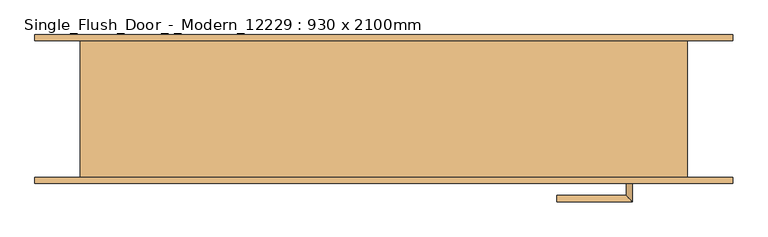
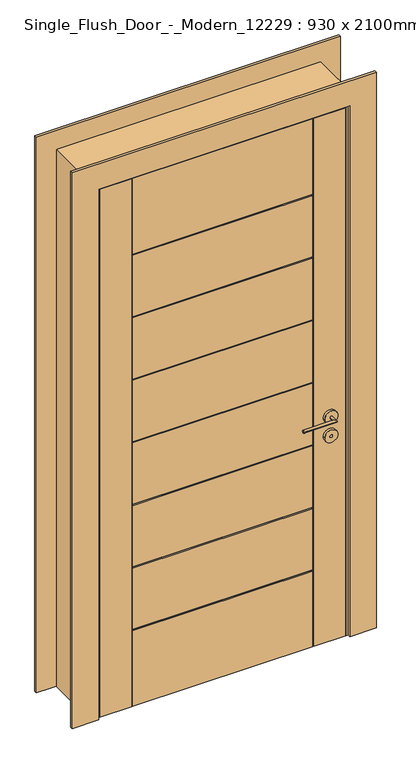
"""IFC4 building model written with IfcOpenShell, lengths in millimetres: door geometry, Single_Flush_Door_-_Modern_12229 : 930 x 2100mm."""

from ifc_helpers import new_model, si_unit, point, frame, frame_2d, origin, place, context, project, spatial, polyline, circle_curve, ellipse_curve, trimmed, segment, composite_curve, outline, extrude, faceted_brep, source, transform, mapped, element, save
from ifc_brep_helpers import plane_surface, cylinder_surface, advanced_brep


def single_flush_door_modern_12229_930_x_2100mm_fac4ccff(model_context):
    return source(origin(), model_context, "Body", "SolidModel", [
        extrude(outline(composite_curve([segment(trimmed(circle_curve(frame_2d((825.0, 405.0)), 25.0), [point((825.0, 380.0))], [point((825.0, 430.0))], False, "CARTESIAN"), True, "CONTINUOUS"), segment(trimmed(circle_curve(frame_2d((825.0, 405.0)), 25.0), [point((825.0, 430.0))], [point((825.0, 380.0))], False, "CARTESIAN"), True, "CONTINUOUS")], self_intersect=False), holes=[composite_curve([segment(trimmed(circle_curve(frame_2d((825.0, 405.0)), 5.0), [point((825.0, 400.0))], [point((825.0, 410.0))], True, "CARTESIAN"), True, "CONTINUOUS"), segment(trimmed(circle_curve(frame_2d((825.0, 405.0)), 5.0), [point((825.0, 410.0))], [point((825.0, 400.0))], True, "CARTESIAN"), True, "CONTINUOUS")], self_intersect=False)]), frame((0.0, -30.0, 0.0), z_axis=(0.0, 1.0, 0.0), x_axis=(0.0, 0.0, 1.0)), (0.0, 0.0, 1.0), 10.0),
        advanced_brep(
        [(410.0, -20.0, 900.0), (400.0, -20.0, 900.0), (410.0, 10.0, 900.0), (400.0, 0.0, 900.0), (285.0, 10.0, 900.0), (285.0, 0.0, 900.0)],
        [
            (0, 1, circle_curve(frame((405.0, -20.0, 900.0), z_axis=(0.0, -1.0, 0.0), x_axis=(-1.0, 0.0, 1.6983196031465473e-12)), 5.0)),
            (1, 0, circle_curve(frame((405.0, -20.0, 900.0), z_axis=(0.0, -1.0, 0.0), x_axis=(-1.0, 0.0, 1.6983196031465473e-12)), 5.0)),
            (0, 2),
            (2, 3, ellipse_curve(frame((405.0, 5.0, 900.0), z_axis=(0.7071067811869033, -0.7071067811861916, -1.2106711776242668e-12), x_axis=(-0.7071067811861915, -0.7071067811869034, 1.1911154383896718e-12)), 7.0710678, 5.0)),
            (3, 1),
            (3, 2, ellipse_curve(frame((405.0, 5.0, 900.0), z_axis=(0.7071067811869033, -0.7071067811861916, -1.2106711776242668e-12), x_axis=(-0.7071067811861915, -0.7071067811869034, 1.1911154383896718e-12)), 7.0710678, 5.0)),
            (4, 5, circle_curve(frame((285.0, 5.0, 900.0), z_axis=(-1.0, 0.0, 1.6983196031465471e-12), x_axis=(0.0, -1.0, 0.0)), 5.0)),
            (5, 4, circle_curve(frame((285.0, 5.0, 900.0), z_axis=(-1.0, 0.0, 1.6983196031465471e-12), x_axis=(0.0, -1.0, 0.0)), 5.0)),
            (2, 4),
            (5, 3),
        ],
        [
            plane_surface(frame((405.0, -20.0, 900.0), z_axis=(0.0, -1.0, 0.0), x_axis=(1.6983196031465542e-12, 0.0, 1.0))),
            cylinder_surface(frame((405.0, -20.0, 900.0), z_axis=(0.0, -1.0, 0.0), x_axis=(-1.0, 0.0, 1.6983196031465473e-12)), 5.0),
            plane_surface(frame((285.0, 5.0, 900.0), z_axis=(-1.0, 0.0, 1.6983196031465473e-12), x_axis=(1.6983196031465542e-12, 0.0, 1.0))),
            cylinder_surface(frame((405.0, 5.0, 900.0), z_axis=(1.0, 0.0, -1.6983196031465471e-12), x_axis=(0.0, -1.0, 0.0)), 5.0),
        ],
        [
            (0, [[1, 2]]),
            (1, [[-1, 3, 4, 5]]),
            (1, [[-2, -5, 6, -3]]),
            (2, [[7, 8]]),
            (3, [[-4, 9, -8, 10]]),
            (3, [[-6, -10, -7, -9]]),
        ],
    ),
        extrude(outline(composite_curve([segment(trimmed(circle_curve(frame_2d((900.0, 405.0)), 25.0), [point((900.0, 380.0))], [point((900.0, 430.0))], False, "CARTESIAN"), True, "CONTINUOUS"), segment(trimmed(circle_curve(frame_2d((900.0, 405.0)), 25.0), [point((900.0, 430.0))], [point((900.0, 380.0))], False, "CARTESIAN"), True, "CONTINUOUS")], self_intersect=False)), frame((0.0, -30.0, 0.0), z_axis=(0.0, 1.0, 0.0), x_axis=(0.0, 0.0, 1.0)), (0.0, 0.0, 1.0), 10.0),
        extrude(outline(composite_curve([segment(trimmed(circle_curve(frame_2d((825.0, 405.0)), 25.0), [point((825.0, 380.0))], [point((825.0, 430.0))], False, "CARTESIAN"), True, "CONTINUOUS"), segment(trimmed(circle_curve(frame_2d((825.0, 405.0)), 25.0), [point((825.0, 430.0))], [point((825.0, 380.0))], False, "CARTESIAN"), True, "CONTINUOUS")], self_intersect=False), holes=[composite_curve([segment(trimmed(circle_curve(frame_2d((825.0, 405.0)), 5.0), [point((825.0, 400.0))], [point((825.0, 410.0))], True, "CARTESIAN"), True, "CONTINUOUS"), segment(trimmed(circle_curve(frame_2d((825.0, 405.0)), 5.0), [point((825.0, 410.0))], [point((825.0, 400.0))], True, "CARTESIAN"), True, "CONTINUOUS")], self_intersect=False)]), frame((0.0, -122.5, 0.0), z_axis=(0.0, 1.0, 0.0), x_axis=(0.0, 0.0, 1.0)), (0.0, 0.0, 1.0), 10.0),
        advanced_brep(
        [(410.0, -122.5, 900.0), (400.0, -122.5, 900.0), (400.0, -142.5, 900.0), (410.0, -152.5, 900.0), (285.0, -152.5, 900.0), (285.0, -142.5, 900.0)],
        [
            (0, 1, circle_curve(frame((405.0, -122.5, 900.0), z_axis=(0.0, 1.0, 0.0), x_axis=(-1.0, 0.0, -1.9708679133145848e-12)), 5.0)),
            (1, 0, circle_curve(frame((405.0, -122.5, 900.0), z_axis=(0.0, 1.0, 0.0), x_axis=(-1.0, 0.0, -1.9708679133145848e-12)), 5.0)),
            (1, 2),
            (2, 3, ellipse_curve(frame((405.0, -147.5, 900.0), z_axis=(0.7071067811869033, 0.7071067811861916, 1.3838361967117316e-12), x_axis=(-0.7071067811861915, 0.7071067811869034, -1.4033919359437145e-12)), 7.0710678, 5.0)),
            (3, 0),
            (3, 2, ellipse_curve(frame((405.0, -147.5, 900.0), z_axis=(0.7071067811869033, 0.7071067811861916, 1.3838361967117316e-12), x_axis=(-0.7071067811861915, 0.7071067811869034, -1.4033919359437145e-12)), 7.0710678, 5.0)),
            (4, 5, circle_curve(frame((285.0, -147.5, 900.0), z_axis=(-1.0, 0.0, -1.9708679133145848e-12), x_axis=(0.0, 1.0, 0.0)), 5.0)),
            (5, 4, circle_curve(frame((285.0, -147.5, 900.0), z_axis=(-1.0, 0.0, -1.9708679133145848e-12), x_axis=(0.0, 1.0, 0.0)), 5.0)),
            (2, 5),
            (4, 3),
        ],
        [
            plane_surface(frame((405.0, -122.5, 900.0), z_axis=(0.0, 1.0, 0.0), x_axis=(-1.970867913314578e-12, 0.0, 1.0))),
            cylinder_surface(frame((405.0, -122.5, 900.0), z_axis=(0.0, 1.0, 0.0), x_axis=(-1.0, 0.0, -1.9708679133145848e-12)), 5.0),
            plane_surface(frame((285.0, -147.5, 900.0), z_axis=(-1.0, 0.0, -1.9708679133145848e-12), x_axis=(-1.970867913314578e-12, 0.0, 1.0))),
            cylinder_surface(frame((405.0, -147.5, 900.0), z_axis=(1.0, 0.0, 1.9708679133145848e-12), x_axis=(0.0, 1.0, 0.0)), 5.0),
        ],
        [
            (0, [[1, 2]]),
            (1, [[3, 4, 5, -2]]),
            (1, [[-5, 6, -3, -1]]),
            (2, [[7, 8]]),
            (3, [[9, -7, 10, -4]]),
            (3, [[-10, -8, -9, -6]]),
        ],
    ),
        extrude(outline(composite_curve([segment(trimmed(circle_curve(frame_2d((900.0, 405.0)), 25.0), [point((900.0, 380.0))], [point((900.0, 430.0))], False, "CARTESIAN"), True, "CONTINUOUS"), segment(trimmed(circle_curve(frame_2d((900.0, 405.0)), 25.0), [point((900.0, 430.0))], [point((900.0, 380.0))], False, "CARTESIAN"), True, "CONTINUOUS")], self_intersect=False)), frame((0.0, -122.5, 0.0), z_axis=(0.0, 1.0, 0.0), x_axis=(0.0, 0.0, 1.0)), (0.0, 0.0, 1.0), 10.0),
        extrude(outline(polyline([(2220.0, -575.0), (0.0, -575.0), (0.0, -475.0), (2120.0, -475.0), (2120.0, 475.0), (0.0, 475.0), (0.0, 575.0), (2220.0, 575.0), (2220.0, -575.0)])), frame((0.0, -122.5, 0.0), z_axis=(0.0, 1.0, 0.0), x_axis=(0.0, 0.0, 1.0)), (0.0, 0.0, 1.0), 10.0),
        extrude(outline(polyline([(2120.0, -475.0), (2120.0, 475.0), (0.0, 475.0), (0.0, 575.0), (2220.0, 575.0), (2220.0, -575.0), (0.0, -575.0), (0.0, -475.0), (2120.0, -475.0)])), frame((0.0, 112.5, 0.0), z_axis=(0.0, 1.0, 0.0), x_axis=(0.0, 0.0, 1.0)), (0.0, 0.0, 1.0), 10.0),
        faceted_brep([(-455.0, 112.5, 0.0), (-455.0, -30.0, 0.0), (-465.0, -30.0, 0.0), (-465.0, -112.5, 0.0), (-500.0, -112.5, 0.0), (-500.0, 112.5, 0.0), (-455.0, 112.5, 2100.0), (-455.0, -30.0, 2100.0), (-345.0, -30.0, 2100.0), (-340.0, -30.0, 2100.0), (340.0, -30.0, 2100.0), (345.0, -30.0, 2100.0), (455.0, -30.0, 2100.0), (455.0, -30.0, 0.0), (465.0, -30.0, 0.0), (465.0, -30.0, 2110.0), (345.0, -30.0, 2110.0), (340.0, -30.0, 2110.0), (-340.0, -30.0, 2110.0), (-345.0, -30.0, 2110.0), (-465.0, -30.0, 2110.0), (-465.0, -112.5, 2110.0), (-345.0, -112.5, 2110.0), (-340.0, -112.5, 2110.0), (340.0, -112.5, 2110.0), (345.0, -112.5, 2110.0), (465.0, -112.5, 2110.0), (465.0, -112.5, 0.0), (500.0, -112.5, 0.0), (500.0, -112.5, 2145.0), (-500.0, -112.5, 2145.0), (-500.0, 112.5, 2145.0), (500.0, 112.5, 2145.0), (500.0, 112.5, 0.0), (455.0, 112.5, 0.0), (455.0, 112.5, 2100.0)], [[[0, 1, 2, 3, 4, 5]], [[1, 0, 6, 7]], [[2, 1, 7, 8, 9, 10, 11, 12, 13, 14, 15, 16, 17, 18, 19, 20]], [[3, 2, 20, 21]], [[4, 3, 21, 22, 23, 24, 25, 26, 27, 28, 29, 30]], [[5, 4, 30, 31]], [[0, 5, 31, 32, 33, 34, 35, 6]], [[13, 12, 35, 34]], [[14, 13, 34, 33, 28, 27]], [[15, 14, 27, 26]], [[29, 28, 33, 32]], [[7, 6, 35, 12, 11, 10, 9, 8]], [[21, 20, 19, 18, 17, 16, 15, 26, 25, 24, 23, 22]], [[30, 29, 32, 31]]]),
        faceted_brep([(465.0, -112.5, 2110.0), (465.0, -30.0, 2110.0), (345.0, -30.0, 2110.0), (345.0, -35.0, 2110.0), (340.0, -35.0, 2110.0), (340.0, -30.0, 2110.0), (-340.0, -30.0, 2110.0), (-340.0, -35.0, 2110.0), (-345.0, -35.0, 2110.0), (-345.0, -30.0, 2110.0), (-465.0, -30.0, 2110.0), (-465.0, -112.5, 2110.0), (-345.0, -112.5, 2110.0), (-345.0, -107.5, 2110.0), (-340.0, -107.5, 2110.0), (-340.0, -112.5, 2110.0), (340.0, -112.5, 2110.0), (340.0, -107.5, 2110.0), (345.0, -107.5, 2110.0), (345.0, -112.5, 2110.0), (-465.0, -112.5, 0.0), (-465.0, -30.0, 0.0), (-345.0, -30.0, 0.0), (-345.0, -35.0, 0.0), (-340.0, -35.0, 0.0), (-340.0, -30.0, 0.0), (340.0, -30.0, 0.0), (340.0, -35.0, 0.0), (345.0, -35.0, 0.0), (345.0, -30.0, 0.0), (465.0, -30.0, 0.0), (465.0, -112.5, 0.0), (345.0, -112.5, 0.0), (345.0, -107.5, 0.0), (340.0, -107.5, 0.0), (340.0, -112.5, 0.0), (-340.0, -112.5, 0.0), (-340.0, -107.5, 0.0), (-345.0, -107.5, 0.0), (-345.0, -112.5, 0.0), (340.0, -30.0, 1807.5), (-340.0, -30.0, 1807.5), (-340.0, -30.0, 302.5), (340.0, -30.0, 302.5), (340.0, -30.0, 1802.5), (340.0, -30.0, 1557.5), (-340.0, -30.0, 1557.5), (-340.0, -30.0, 1802.5), (340.0, -30.0, 1552.5), (340.0, -30.0, 1307.5), (-340.0, -30.0, 1307.5), (-340.0, -30.0, 1552.5), (340.0, -30.0, 1302.5), (340.0, -30.0, 1057.5), (-340.0, -30.0, 1057.5), (-340.0, -30.0, 1302.5), (340.0, -30.0, 1052.5), (340.0, -30.0, 807.5), (-340.0, -30.0, 807.5), (-340.0, -30.0, 1052.5), (340.0, -30.0, 802.5), (340.0, -30.0, 557.5), (-340.0, -30.0, 557.5), (-340.0, -30.0, 802.5), (340.0, -30.0, 552.5), (340.0, -30.0, 307.5), (-340.0, -30.0, 307.5), (-340.0, -30.0, 552.5), (-340.0, -112.5, 1807.5), (340.0, -112.5, 1807.5), (340.0, -112.5, 302.5), (-340.0, -112.5, 302.5), (-340.0, -112.5, 1802.5), (-340.0, -112.5, 1557.5), (340.0, -112.5, 1557.5), (340.0, -112.5, 1802.5), (-340.0, -112.5, 1552.5), (-340.0, -112.5, 1307.5), (340.0, -112.5, 1307.5), (340.0, -112.5, 1552.5), (-340.0, -112.5, 1302.5), (-340.0, -112.5, 1057.5), (340.0, -112.5, 1057.5), (340.0, -112.5, 1302.5), (-340.0, -112.5, 1052.5), (-340.0, -112.5, 807.5), (340.0, -112.5, 807.5), (340.0, -112.5, 1052.5), (-340.0, -112.5, 802.5), (-340.0, -112.5, 557.5), (340.0, -112.5, 557.5), (340.0, -112.5, 802.5), (-340.0, -112.5, 552.5), (-340.0, -112.5, 307.5), (340.0, -112.5, 307.5), (340.0, -112.5, 552.5), (-340.0, -107.5, 302.5), (340.0, -107.5, 302.5), (340.0, -107.5, 1807.5), (-340.0, -107.5, 1807.5), (-340.0, -107.5, 1802.5), (340.0, -107.5, 1802.5), (340.0, -107.5, 1557.5), (-340.0, -107.5, 1557.5), (-340.0, -107.5, 1552.5), (340.0, -107.5, 1552.5), (340.0, -107.5, 1307.5), (-340.0, -107.5, 1307.5), (-340.0, -107.5, 1302.5), (340.0, -107.5, 1302.5), (340.0, -107.5, 1057.5), (-340.0, -107.5, 1057.5), (-340.0, -107.5, 1052.5), (340.0, -107.5, 1052.5), (340.0, -107.5, 807.5), (-340.0, -107.5, 807.5), (-340.0, -107.5, 802.5), (340.0, -107.5, 802.5), (340.0, -107.5, 557.5), (-340.0, -107.5, 557.5), (-340.0, -107.5, 552.5), (340.0, -107.5, 552.5), (340.0, -107.5, 307.5), (-340.0, -107.5, 307.5), (340.0, -35.0, 302.5), (-340.0, -35.0, 302.5), (-340.0, -35.0, 1807.5), (340.0, -35.0, 1807.5), (340.0, -35.0, 1557.5), (340.0, -35.0, 1802.5), (-340.0, -35.0, 1802.5), (-340.0, -35.0, 1557.5), (340.0, -35.0, 1307.5), (340.0, -35.0, 1552.5), (-340.0, -35.0, 1552.5), (-340.0, -35.0, 1307.5), (340.0, -35.0, 1057.5), (340.0, -35.0, 1302.5), (-340.0, -35.0, 1302.5), (-340.0, -35.0, 1057.5), (340.0, -35.0, 807.5), (340.0, -35.0, 1052.5), (-340.0, -35.0, 1052.5), (-340.0, -35.0, 807.5), (340.0, -35.0, 557.5), (340.0, -35.0, 802.5), (-340.0, -35.0, 802.5), (-340.0, -35.0, 557.5), (340.0, -35.0, 307.5), (340.0, -35.0, 552.5), (-340.0, -35.0, 552.5), (-340.0, -35.0, 307.5)], [[[0, 1, 2, 3, 4, 5, 6, 7, 8, 9, 10, 11, 12, 13, 14, 15, 16, 17, 18, 19]], [[20, 21, 22, 23, 24, 25, 26, 27, 28, 29, 30, 31, 32, 33, 34, 35, 36, 37, 38, 39]], [[1, 0, 31, 30]], [[6, 5, 40, 41]], [[26, 25, 42, 43]], [[1, 30, 29, 2]], [[21, 10, 9, 22]], [[44, 45, 46, 47]], [[48, 49, 50, 51]], [[52, 53, 54, 55]], [[56, 57, 58, 59]], [[60, 61, 62, 63]], [[64, 65, 66, 67]], [[11, 10, 21, 20]], [[16, 15, 68, 69]], [[36, 35, 70, 71]], [[31, 0, 19, 32]], [[11, 20, 39, 12]], [[72, 73, 74, 75]], [[76, 77, 78, 79]], [[80, 81, 82, 83]], [[84, 85, 86, 87]], [[88, 89, 90, 91]], [[92, 93, 94, 95]], [[13, 38, 37, 96, 97, 34, 33, 18, 17, 98, 99, 14], [100, 101, 102, 103], [104, 105, 106, 107], [108, 109, 110, 111], [112, 113, 114, 115], [116, 117, 118, 119], [120, 121, 122, 123]], [[15, 14, 99, 68]], [[37, 36, 71, 96]], [[73, 72, 100, 103]], [[77, 76, 104, 107]], [[81, 80, 108, 111]], [[85, 84, 112, 115]], [[89, 88, 116, 119]], [[93, 92, 120, 123]], [[38, 13, 12, 39]], [[18, 33, 32, 19]], [[17, 16, 69, 98]], [[35, 34, 97, 70]], [[75, 74, 102, 101]], [[79, 78, 106, 105]], [[83, 82, 110, 109]], [[87, 86, 114, 113]], [[91, 90, 118, 117]], [[95, 94, 122, 121]], [[101, 100, 72, 75]], [[99, 98, 69, 68]], [[105, 104, 76, 79]], [[103, 102, 74, 73]], [[109, 108, 80, 83]], [[107, 106, 78, 77]], [[113, 112, 84, 87]], [[111, 110, 82, 81]], [[117, 116, 88, 91]], [[115, 114, 86, 85]], [[121, 120, 92, 95]], [[119, 118, 90, 89]], [[97, 96, 71, 70]], [[123, 122, 94, 93]], [[3, 28, 27, 124, 125, 24, 23, 8, 7, 126, 127, 4], [128, 129, 130, 131], [132, 133, 134, 135], [136, 137, 138, 139], [140, 141, 142, 143], [144, 145, 146, 147], [148, 149, 150, 151]], [[5, 4, 127, 40]], [[27, 26, 43, 124]], [[45, 44, 129, 128]], [[49, 48, 133, 132]], [[53, 52, 137, 136]], [[57, 56, 141, 140]], [[61, 60, 145, 144]], [[65, 64, 149, 148]], [[28, 3, 2, 29]], [[8, 23, 22, 9]], [[7, 6, 41, 126]], [[25, 24, 125, 42]], [[47, 46, 131, 130]], [[51, 50, 135, 134]], [[55, 54, 139, 138]], [[59, 58, 143, 142]], [[63, 62, 147, 146]], [[67, 66, 151, 150]], [[127, 126, 41, 40]], [[130, 129, 44, 47]], [[128, 131, 46, 45]], [[134, 133, 48, 51]], [[132, 135, 50, 49]], [[138, 137, 52, 55]], [[136, 139, 54, 53]], [[142, 141, 56, 59]], [[140, 143, 58, 57]], [[146, 145, 60, 63]], [[144, 147, 62, 61]], [[150, 149, 64, 67]], [[148, 151, 66, 65]], [[125, 124, 43, 42]]]),
    ])


if __name__ == "__main__":
    model = new_model("IFC4")
    model_context = context("Model", 3, world=origin())
    ifc_project = project(units=[si_unit("LENGTHUNIT", "METRE", prefix="MILLI")], contexts=[model_context])
    site = spatial("IfcSite", under=ifc_project)
    building = spatial("IfcBuilding", under=site)
    placement = place(None, origin())
    single_flush_door_modern_12229_930_x_2100mm_shape = single_flush_door_modern_12229_930_x_2100mm_fac4ccff(model_context)
    element("IfcDoor", 1, ObjectType="Single_Flush_Door_-_Modern_12229 : 930 x 2100mm", at=placement, inside=building, context=model_context, shape_type="MappedRepresentation", body=[
        mapped(single_flush_door_modern_12229_930_x_2100mm_shape, transform((0.0, 0.0, 0.0), x_axis=(1.0, 0.0, 0.0), y_axis=(0.0, 1.0, 0.0), z_axis=(0.0, 0.0, 1.0))),
    ])
    save(model, "model.ifc")

# Revit data of these elements
# Type "Single_Flush_Door_-_Modern_12229 : 930 x 2100mm"
#   Type Mark = "50"
#   Description = "HWD FRAMED & PANELLED SINGLE DOOR"
#   Analytic Construction = "<None>"
#   Thickness = 45 mm
#   Rough Width = 1000 mm
#   Rough Height = 2145 mm
#   Frame Projection Ext. = 10 mm
#   Frame Projection Int. = 10 mm
#   Frame Width = 75 mm
#   Height = 2100 mm
#   Width = 930 mm
#   Define Thermal Properties by = 1
#   Jamb Material = Window Frame
#   Door Material = Window Frame
#   Function = (empty or 0)
#   Wall Closure = (empty or 0)
#   Assembly Code = ""
# Element 1 (IfcDoor, "Single_Flush_Door_-_Modern_12229 : 930 x 2100mm")
#   Materials on its faces: "Window Frame"
# Materials
#   "Window Frame": colour RGB 249 249 249, transparency 0, Keynote = "L10", Cost = 0
